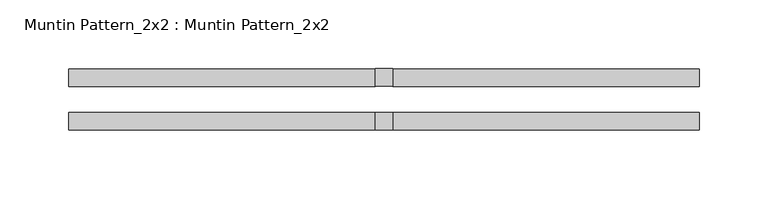
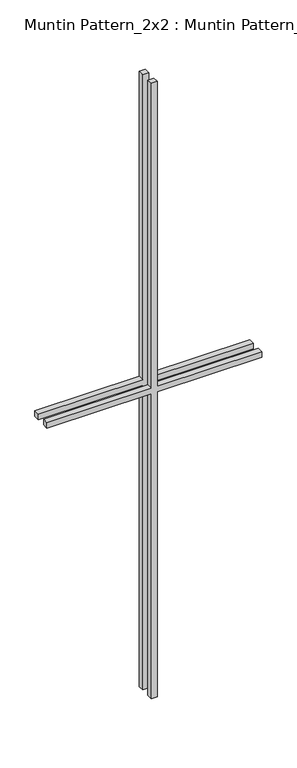
"""IFC4 building model written with IfcOpenShell, lengths in millimetres: proxy geometry, Muntin Pattern_2x2 : Muntin Pattern_2x2."""

from ifc_helpers import new_model, si_unit, frame, origin, place, context, project, spatial, polyline, outline, extrude, source, transform, mapped, element, save


def muntin_pattern_2x2_muntin_pattern_2x2_32baafd4(model_context):
    return source(origin(), model_context, "Body", "SweptSolid", [
        extrude(outline(polyline([(698.5, -6.35), (698.5, -228.6), (685.8, -228.6), (685.8, -6.35), (0.0, -6.35), (0.0, 6.35), (685.8, 6.35), (685.8, 228.6), (698.5, 228.6), (698.5, 6.35), (1384.3, 6.35), (1384.3, -6.35), (698.5, -6.35)])), frame((0.0, -22.225, 0.0), z_axis=(0.0, 1.0, 0.0), x_axis=(0.0, 0.0, 1.0)), (0.0, 0.0, 1.0), 12.7),
        extrude(outline(polyline([(698.5, -6.35), (698.5, -228.6), (685.8, -228.6), (685.8, -6.35), (0.0, -6.35), (0.0, 6.35), (685.8, 6.35), (685.8, 228.6), (698.5, 228.6), (698.5, 6.35), (1384.3, 6.35), (1384.3, -6.35), (698.5, -6.35)])), frame((0.0, 9.525, 0.0), z_axis=(0.0, 1.0, 0.0), x_axis=(0.0, 0.0, 1.0)), (0.0, 0.0, 1.0), 12.7),
    ])


if __name__ == "__main__":
    model = new_model("IFC4")
    model_context = context("Model", 3, world=origin())
    ifc_project = project(units=[si_unit("LENGTHUNIT", "METRE", prefix="MILLI")], contexts=[model_context])
    site = spatial("IfcSite", under=ifc_project)
    building = spatial("IfcBuilding", under=site)
    placement = place(None, origin())
    muntin_pattern_2x2_muntin_pattern_2x2_shape = muntin_pattern_2x2_muntin_pattern_2x2_32baafd4(model_context)
    element("IfcBuildingElementProxy", 1, Name="Muntin Pattern_2x2 : Muntin Pattern_2x2", ObjectType="Muntin Pattern_2x2 : Muntin Pattern_2x2", at=placement, inside=building, context=model_context, shape_type="MappedRepresentation", body=[
        mapped(muntin_pattern_2x2_muntin_pattern_2x2_shape, transform((0.0, 0.0, 0.0), x_axis=(1.0, 0.0, 0.0), y_axis=(0.0, 1.0, 0.0), z_axis=(0.0, 0.0, 1.0))),
    ])
    save(model, "model.ifc")

# Revit data of these elements
# Type "Muntin Pattern_2x2 : Muntin Pattern_2x2"
#   Width [instance default] = 4' - 0"
#   Thickness = 0' - 0 1/2"
#   Height [instance default] = 4' - 0"
#   Distance = 0' - 0 3/4"
#   Interior Material [instance default] = none
#   Exterior Material [instance default] = none
#   Default Elevation = 0
# Element 1 (IfcBuildingElementProxy, "Muntin Pattern_2x2 : Muntin Pattern_2x2")
#   Width = 1' - 6"
#   Height = 4' - 6 1/2"
#   Interior Material = Wood - Stained
#   Exterior Material = Clad - White
#   Materials on its faces: "Clad - White", "Wood - Stained"
# Materials
#   "Clad - White": class "Wood", colour RGB 30 30 30, transparency 0, Cost = 0
#   "Wood - Stained": class "Wood", colour RGB 224 178 126, transparency 0, Cost = 0
